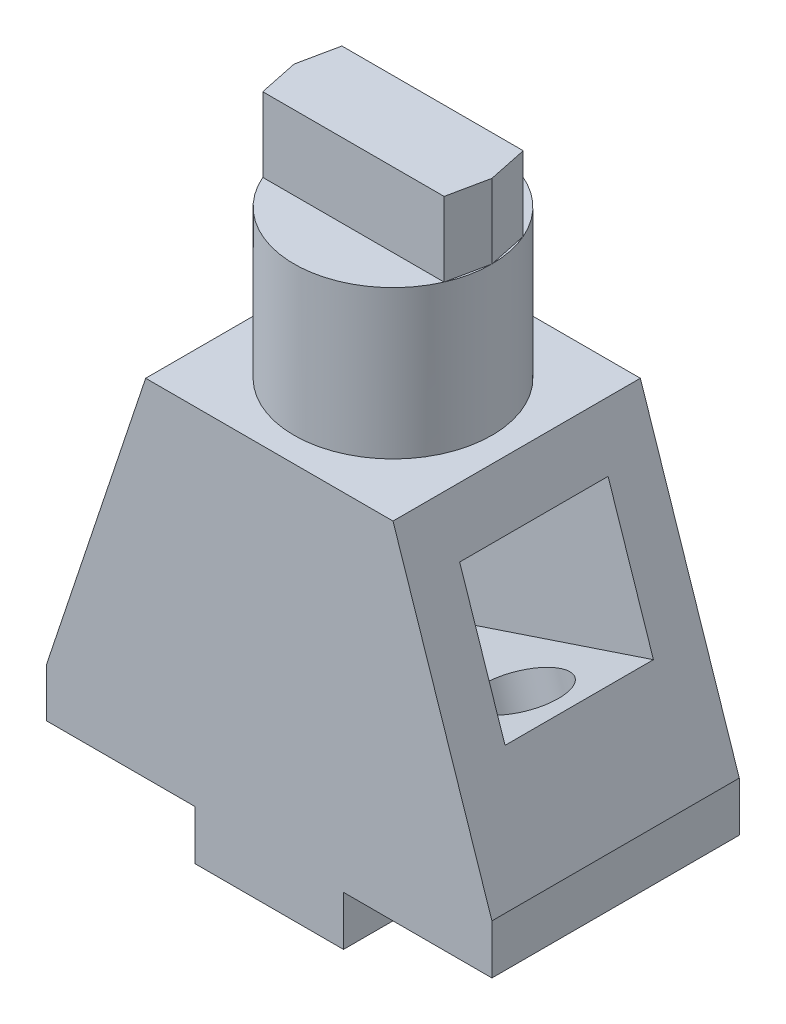
ISO-10303-21;
HEADER;
FILE_DESCRIPTION(('STEP AP214'),'2;1');
FILE_NAME('part.step','',(''),(''),'','','');
FILE_SCHEMA(('AUTOMOTIVE_DESIGN { 1 0 10303 214 1 1 1 1 }'));
ENDSEC;
DATA;
#1=APPLICATION_CONTEXT('core data for automotive mechanical design processes');
#2=APPLICATION_PROTOCOL_DEFINITION('international standard','automotive_design',2000,#1);
#3=PRODUCT_CONTEXT('',#1,'mechanical');
#4=PRODUCT('Part','Part','',(#3));
#5=PRODUCT_RELATED_PRODUCT_CATEGORY('part','',(#4));
#6=PRODUCT_DEFINITION_FORMATION('','',#4);
#7=PRODUCT_DEFINITION_CONTEXT('part definition',#1,'design');
#8=PRODUCT_DEFINITION('design','',#6,#7);
#9=PRODUCT_DEFINITION_SHAPE('','',#8);
#10=(LENGTH_UNIT() NAMED_UNIT(*) SI_UNIT(.MILLI.,.METRE.));
#11=(NAMED_UNIT(*) PLANE_ANGLE_UNIT() SI_UNIT($,.RADIAN.));
#12=(NAMED_UNIT(*) SI_UNIT($,.STERADIAN.) SOLID_ANGLE_UNIT());
#13=UNCERTAINTY_MEASURE_WITH_UNIT(LENGTH_MEASURE(1.E-05),#10,'distance_accuracy_value','');
#14=(GEOMETRIC_REPRESENTATION_CONTEXT(3) GLOBAL_UNCERTAINTY_ASSIGNED_CONTEXT((#13)) GLOBAL_UNIT_ASSIGNED_CONTEXT((#10,
#11,#12)) REPRESENTATION_CONTEXT('',''));
#15=CARTESIAN_POINT('',(0.,0.,0.));
#16=DIRECTION('',(0.,0.,1.));
#17=DIRECTION('',(1.,0.,0.));
#18=AXIS2_PLACEMENT_3D('',#15,#16,#17);
#19=CARTESIAN_POINT('',(45.,100.,-25.));
#20=DIRECTION('',(0.,1.,0.));
#21=DIRECTION('',(0.,0.,1.));
#22=AXIS2_PLACEMENT_3D('',#19,#20,#21);
#23=PLANE('',#22);
#24=DIRECTION('',(0.20430964368922,0.,0.978906312930703));
#25=VECTOR('',#24,1.);
#26=CARTESIAN_POINT('',(26.6696972201766,100.,-17.));
#27=LINE('',#26,#25);
#28=CARTESIAN_POINT('',(25.,100.,-25.));
#29=VERTEX_POINT('',#28);
#30=CARTESIAN_POINT('',(26.6696972201766,100.,-17.));
#31=VERTEX_POINT('',#30);
#32=EDGE_CURVE('E65',#29,#31,#27,.T.);
#33=ORIENTED_EDGE('',*,*,#32,.F.);
#34=CARTESIAN_POINT('',(45.,100.,-25.));
#35=DIRECTION('',(0.,1.,0.));
#36=DIRECTION('',(0.,0.,1.));
#37=AXIS2_PLACEMENT_3D('',#34,#35,#36);
#38=CIRCLE('',#37,20.);
#39=EDGE_CURVE('E209',#29,#31,#38,.T.);
#40=ORIENTED_EDGE('',*,*,#39,.T.);
#41=EDGE_LOOP('',(#33,#40));
#42=FACE_BOUND('',#41,.T.);
#43=ADVANCED_FACE('F39',(#42),#23,.T.);
#44=DIRECTION('',(-0.20430964368922,0.,0.978906312930703));
#45=VECTOR('',#44,1.);
#46=CARTESIAN_POINT('',(25.,100.,-25.));
#47=LINE('',#46,#45);
#48=CARTESIAN_POINT('',(26.6696972201766,100.,-33.));
#49=VERTEX_POINT('',#48);
#50=EDGE_CURVE('E202',#49,#29,#47,.T.);
#51=ORIENTED_EDGE('',*,*,#50,.F.);
#52=EDGE_CURVE('E476',#49,#29,#38,.T.);
#53=ORIENTED_EDGE('',*,*,#52,.T.);
#54=EDGE_LOOP('',(#51,#53));
#55=FACE_BOUND('',#54,.T.);
#56=ADVANCED_FACE('F410',(#55),#23,.T.);
#57=DIRECTION('',(-1.,0.,0.));
#58=VECTOR('',#57,1.);
#59=CARTESIAN_POINT('',(26.6696972201766,100.,-33.));
#60=LINE('',#59,#58);
#61=CARTESIAN_POINT('',(63.3303027798234,100.,-33.));
#62=VERTEX_POINT('',#61);
#63=EDGE_CURVE('E457',#62,#49,#60,.T.);
#64=ORIENTED_EDGE('',*,*,#63,.F.);
#65=EDGE_CURVE('E483',#62,#49,#38,.T.);
#66=ORIENTED_EDGE('',*,*,#65,.T.);
#67=EDGE_LOOP('',(#64,#66));
#68=FACE_BOUND('',#67,.T.);
#69=ADVANCED_FACE('F411',(#68),#23,.T.);
#70=DIRECTION('',(-0.20430964368922,0.,-0.978906312930703));
#71=VECTOR('',#70,1.);
#72=CARTESIAN_POINT('',(63.3303027798234,100.,-33.));
#73=LINE('',#72,#71);
#74=CARTESIAN_POINT('',(65.,100.,-25.));
#75=VERTEX_POINT('',#74);
#76=EDGE_CURVE('E438',#75,#62,#73,.T.);
#77=ORIENTED_EDGE('',*,*,#76,.F.);
#78=EDGE_CURVE('E217',#75,#62,#38,.T.);
#79=ORIENTED_EDGE('',*,*,#78,.T.);
#80=EDGE_LOOP('',(#77,#79));
#81=FACE_BOUND('',#80,.T.);
#82=ADVANCED_FACE('F426',(#81),#23,.T.);
#83=DIRECTION('',(0.20430964368922,0.,-0.978906312930703));
#84=VECTOR('',#83,1.);
#85=CARTESIAN_POINT('',(65.,100.,-25.));
#86=LINE('',#85,#84);
#87=CARTESIAN_POINT('',(63.3303027798234,100.,-17.));
#88=VERTEX_POINT('',#87);
#89=EDGE_CURVE('E434',#88,#75,#86,.T.);
#90=ORIENTED_EDGE('',*,*,#89,.F.);
#91=EDGE_CURVE('E215',#88,#75,#38,.T.);
#92=ORIENTED_EDGE('',*,*,#91,.T.);
#93=EDGE_LOOP('',(#90,#92));
#94=FACE_BOUND('',#93,.T.);
#95=ADVANCED_FACE('F420',(#94),#23,.T.);
#96=CARTESIAN_POINT('',(0.,10.,-50.));
#97=DIRECTION('',(-1.,0.,0.));
#98=DIRECTION('',(0.,0.,1.));
#99=AXIS2_PLACEMENT_3D('',#96,#97,#98);
#100=PLANE('',#99);
#101=DIRECTION('',(0.,1.,0.));
#102=VECTOR('',#101,1.);
#103=CARTESIAN_POINT('',(0.,10.,-10.));
#104=LINE('',#103,#102);
#105=CARTESIAN_POINT('',(0.,4.50296453108829,-10.));
#106=VERTEX_POINT('',#105);
#107=CARTESIAN_POINT('',(0.,10.,-10.));
#108=VERTEX_POINT('',#107);
#109=EDGE_CURVE('E246',#106,#108,#104,.T.);
#110=ORIENTED_EDGE('',*,*,#109,.F.);
#111=DIRECTION('',(0.,0.,1.));
#112=VECTOR('',#111,1.);
#113=CARTESIAN_POINT('',(0.,4.50296453108829,-50.));
#114=LINE('',#113,#112);
#115=CARTESIAN_POINT('',(0.,4.50296453108829,-40.));
#116=VERTEX_POINT('',#115);
#117=EDGE_CURVE('E249',#116,#106,#114,.T.);
#118=ORIENTED_EDGE('',*,*,#117,.F.);
#119=DIRECTION('',(0.,-1.,0.));
#120=VECTOR('',#119,1.);
#121=CARTESIAN_POINT('',(0.,10.,-40.));
#122=LINE('',#121,#120);
#123=CARTESIAN_POINT('',(0.,10.,-40.));
#124=VERTEX_POINT('',#123);
#125=EDGE_CURVE('E241',#124,#116,#122,.T.);
#126=ORIENTED_EDGE('',*,*,#125,.F.);
#127=DIRECTION('',(0.,0.,1.));
#128=VECTOR('',#127,1.);
#129=CARTESIAN_POINT('',(0.,10.,-50.));
#130=LINE('',#129,#128);
#131=CARTESIAN_POINT('',(0.,10.,-50.));
#132=VERTEX_POINT('',#131);
#133=EDGE_CURVE('E48',#132,#124,#130,.T.);
#134=ORIENTED_EDGE('',*,*,#133,.F.);
#135=DIRECTION('',(0.,-1.,0.));
#136=VECTOR('',#135,1.);
#137=CARTESIAN_POINT('',(0.,10.,-50.));
#138=LINE('',#137,#136);
#139=CARTESIAN_POINT('',(0.,0.,-50.));
#140=VERTEX_POINT('',#139);
#141=EDGE_CURVE('E251',#132,#140,#138,.T.);
#142=ORIENTED_EDGE('',*,*,#141,.T.);
#143=DIRECTION('',(0.,0.,1.));
#144=VECTOR('',#143,1.);
#145=CARTESIAN_POINT('',(0.,0.,-50.));
#146=LINE('',#145,#144);
#147=CARTESIAN_POINT('',(0.,0.,0.));
#148=VERTEX_POINT('',#147);
#149=EDGE_CURVE('E43',#140,#148,#146,.T.);
#150=ORIENTED_EDGE('',*,*,#149,.T.);
#151=DIRECTION('',(0.,-1.,0.));
#152=VECTOR('',#151,1.);
#153=CARTESIAN_POINT('',(0.,10.,0.));
#154=LINE('',#153,#152);
#155=CARTESIAN_POINT('',(0.,10.,0.));
#156=VERTEX_POINT('',#155);
#157=EDGE_CURVE('E252',#156,#148,#154,.T.);
#158=ORIENTED_EDGE('',*,*,#157,.F.);
#159=EDGE_CURVE('E314',#108,#156,#130,.T.);
#160=ORIENTED_EDGE('',*,*,#159,.F.);
#161=EDGE_LOOP('',(#110,#118,#126,#134,#142,#150,#158,#160));
#162=FACE_BOUND('',#161,.T.);
#163=ADVANCED_FACE('F41',(#162),#100,.T.);
#164=CARTESIAN_POINT('',(20.,70.,-50.));
#165=DIRECTION('',(-0.948683298050514,0.316227766016838,0.));
#166=DIRECTION('',(-0.316227766016838,-0.948683298050514,0.));
#167=AXIS2_PLACEMENT_3D('',#164,#165,#166);
#168=PLANE('',#167);
#169=DIRECTION('',(0.316227766016838,0.948683298050514,0.));
#170=VECTOR('',#169,1.);
#171=CARTESIAN_POINT('',(20.,70.,-10.));
#172=LINE('',#171,#170);
#173=CARTESIAN_POINT('',(9.40186821726848,38.2056046518055,-10.));
#174=VERTEX_POINT('',#173);
#175=EDGE_CURVE('E248',#108,#174,#172,.T.);
#176=ORIENTED_EDGE('',*,*,#175,.F.);
#177=ORIENTED_EDGE('',*,*,#159,.T.);
#178=DIRECTION('',(-0.316227766016838,-0.948683298050514,0.));
#179=VECTOR('',#178,1.);
#180=CARTESIAN_POINT('',(20.,70.,0.));
#181=LINE('',#180,#179);
#182=CARTESIAN_POINT('',(20.,70.,0.));
#183=VERTEX_POINT('',#182);
#184=EDGE_CURVE('E260',#183,#156,#181,.T.);
#185=ORIENTED_EDGE('',*,*,#184,.F.);
#186=DIRECTION('',(0.,0.,1.));
#187=VECTOR('',#186,1.);
#188=CARTESIAN_POINT('',(20.,70.,-50.));
#189=LINE('',#188,#187);
#190=CARTESIAN_POINT('',(20.,70.,-50.));
#191=VERTEX_POINT('',#190);
#192=EDGE_CURVE('E312',#191,#183,#189,.T.);
#193=ORIENTED_EDGE('',*,*,#192,.F.);
#194=DIRECTION('',(-0.316227766016838,-0.948683298050514,0.));
#195=VECTOR('',#194,1.);
#196=CARTESIAN_POINT('',(20.,70.,-50.));
#197=LINE('',#196,#195);
#198=EDGE_CURVE('E281',#191,#132,#197,.T.);
#199=ORIENTED_EDGE('',*,*,#198,.T.);
#200=ORIENTED_EDGE('',*,*,#133,.T.);
#201=DIRECTION('',(-0.316227766016838,-0.948683298050514,0.));
#202=VECTOR('',#201,1.);
#203=CARTESIAN_POINT('',(20.,70.,-40.));
#204=LINE('',#203,#202);
#205=CARTESIAN_POINT('',(9.40186821726847,38.2056046518054,-40.));
#206=VERTEX_POINT('',#205);
#207=EDGE_CURVE('E231',#206,#124,#204,.T.);
#208=ORIENTED_EDGE('',*,*,#207,.F.);
#209=DIRECTION('',(0.,0.,-1.));
#210=VECTOR('',#209,1.);
#211=CARTESIAN_POINT('',(9.40186821726848,38.2056046518055,-50.));
#212=LINE('',#211,#210);
#213=EDGE_CURVE('E242',#174,#206,#212,.T.);
#214=ORIENTED_EDGE('',*,*,#213,.F.);
#215=EDGE_LOOP('',(#176,#177,#185,#193,#199,#200,#208,#214));
#216=FACE_BOUND('',#215,.T.);
#217=ADVANCED_FACE('F344',(#216),#168,.T.);
#218=CARTESIAN_POINT('',(70.,70.,-50.));
#219=DIRECTION('',(0.,1.,0.));
#220=DIRECTION('',(0.,0.,1.));
#221=AXIS2_PLACEMENT_3D('',#218,#219,#220);
#222=PLANE('',#221);
#223=CARTESIAN_POINT('',(45.,70.,-25.));
#224=DIRECTION('',(0.,1.,0.));
#225=DIRECTION('',(0.,0.,1.));
#226=AXIS2_PLACEMENT_3D('',#223,#224,#225);
#227=CIRCLE('',#226,20.);
#228=CARTESIAN_POINT('',(45.,70.,-4.99999999999999));
#229=VERTEX_POINT('',#228);
#230=EDGE_CURVE('E11',#229,#229,#227,.T.);
#231=ORIENTED_EDGE('',*,*,#230,.F.);
#232=EDGE_LOOP('',(#231));
#233=FACE_BOUND('',#232,.T.);
#234=DIRECTION('',(-1.,0.,0.));
#235=VECTOR('',#234,1.);
#236=CARTESIAN_POINT('',(70.,70.,0.));
#237=LINE('',#236,#235);
#238=CARTESIAN_POINT('',(70.,70.,0.));
#239=VERTEX_POINT('',#238);
#240=EDGE_CURVE('E307',#239,#183,#237,.T.);
#241=ORIENTED_EDGE('',*,*,#240,.F.);
#242=DIRECTION('',(0.,0.,1.));
#243=VECTOR('',#242,1.);
#244=CARTESIAN_POINT('',(70.,70.,-50.));
#245=LINE('',#244,#243);
#246=CARTESIAN_POINT('',(70.,70.,-50.));
#247=VERTEX_POINT('',#246);
#248=EDGE_CURVE('E320',#247,#239,#245,.T.);
#249=ORIENTED_EDGE('',*,*,#248,.F.);
#250=DIRECTION('',(-1.,0.,0.));
#251=VECTOR('',#250,1.);
#252=CARTESIAN_POINT('',(70.,70.,-50.));
#253=LINE('',#252,#251);
#254=EDGE_CURVE('E279',#247,#191,#253,.T.);
#255=ORIENTED_EDGE('',*,*,#254,.T.);
#256=ORIENTED_EDGE('',*,*,#192,.T.);
#257=EDGE_LOOP('',(#241,#249,#255,#256));
#258=FACE_BOUND('',#257,.T.);
#259=ADVANCED_FACE('F393',(#233,#258),#222,.T.);
#260=CARTESIAN_POINT('',(90.,10.,-50.));
#261=DIRECTION('',(0.948683298050514,0.316227766016838,0.));
#262=DIRECTION('',(-0.316227766016838,0.948683298050514,0.));
#263=AXIS2_PLACEMENT_3D('',#260,#261,#262);
#264=PLANE('',#263);
#265=DIRECTION('',(0.,0.,-1.));
#266=VECTOR('',#265,1.);
#267=CARTESIAN_POINT('',(82.6491106406736,32.0526680779795,-40.));
#268=LINE('',#267,#266);
#269=CARTESIAN_POINT('',(82.6491106406736,32.0526680779795,-10.));
#270=VERTEX_POINT('',#269);
#271=CARTESIAN_POINT('',(82.6491106406736,32.0526680779793,-40.));
#272=VERTEX_POINT('',#271);
#273=EDGE_CURVE('E220',#270,#272,#268,.T.);
#274=ORIENTED_EDGE('',*,*,#273,.F.);
#275=DIRECTION('',(0.316227766016837,-0.948683298050514,0.));
#276=VECTOR('',#275,1.);
#277=CARTESIAN_POINT('',(82.6491106406736,32.0526680779795,-10.));
#278=LINE('',#277,#276);
#279=CARTESIAN_POINT('',(73.4785054261853,59.5644837214444,-10.));
#280=VERTEX_POINT('',#279);
#281=EDGE_CURVE('E230',#280,#270,#278,.T.);
#282=ORIENTED_EDGE('',*,*,#281,.F.);
#283=DIRECTION('',(0.,0.,1.));
#284=VECTOR('',#283,1.);
#285=CARTESIAN_POINT('',(73.4785054261853,59.5644837214444,-10.));
#286=LINE('',#285,#284);
#287=CARTESIAN_POINT('',(73.4785054261853,59.5644837214444,-40.));
#288=VERTEX_POINT('',#287);
#289=EDGE_CURVE('E221',#288,#280,#286,.T.);
#290=ORIENTED_EDGE('',*,*,#289,.F.);
#291=DIRECTION('',(-0.316227766016837,0.948683298050514,0.));
#292=VECTOR('',#291,1.);
#293=CARTESIAN_POINT('',(73.4785054261853,59.5644837214444,-40.));
#294=LINE('',#293,#292);
#295=EDGE_CURVE('E222',#272,#288,#294,.T.);
#296=ORIENTED_EDGE('',*,*,#295,.F.);
#297=EDGE_LOOP('',(#274,#282,#290,#296));
#298=FACE_BOUND('',#297,.T.);
#299=DIRECTION('',(-0.316227766016838,0.948683298050514,0.));
#300=VECTOR('',#299,1.);
#301=CARTESIAN_POINT('',(90.,10.,0.));
#302=LINE('',#301,#300);
#303=CARTESIAN_POINT('',(90.,10.,0.));
#304=VERTEX_POINT('',#303);
#305=EDGE_CURVE('E302',#304,#239,#302,.T.);
#306=ORIENTED_EDGE('',*,*,#305,.F.);
#307=DIRECTION('',(0.,0.,1.));
#308=VECTOR('',#307,1.);
#309=CARTESIAN_POINT('',(90.,10.,-50.));
#310=LINE('',#309,#308);
#311=CARTESIAN_POINT('',(90.,10.,-50.));
#312=VERTEX_POINT('',#311);
#313=EDGE_CURVE('E317',#312,#304,#310,.T.);
#314=ORIENTED_EDGE('',*,*,#313,.F.);
#315=DIRECTION('',(-0.316227766016838,0.948683298050514,0.));
#316=VECTOR('',#315,1.);
#317=CARTESIAN_POINT('',(90.,10.,-50.));
#318=LINE('',#317,#316);
#319=EDGE_CURVE('E274',#312,#247,#318,.T.);
#320=ORIENTED_EDGE('',*,*,#319,.T.);
#321=ORIENTED_EDGE('',*,*,#248,.T.);
#322=EDGE_LOOP('',(#306,#314,#320,#321));
#323=FACE_BOUND('',#322,.T.);
#324=ADVANCED_FACE('F361',(#298,#323),#264,.T.);
#325=CARTESIAN_POINT('',(90.,0.,-50.));
#326=DIRECTION('',(1.,0.,0.));
#327=DIRECTION('',(0.,0.,-1.));
#328=AXIS2_PLACEMENT_3D('',#325,#326,#327);
#329=PLANE('',#328);
#330=DIRECTION('',(0.,1.,0.));
#331=VECTOR('',#330,1.);
#332=CARTESIAN_POINT('',(90.,0.,0.));
#333=LINE('',#332,#331);
#334=CARTESIAN_POINT('',(90.,0.,0.));
#335=VERTEX_POINT('',#334);
#336=EDGE_CURVE('E303',#335,#304,#333,.T.);
#337=ORIENTED_EDGE('',*,*,#336,.F.);
#338=DIRECTION('',(0.,0.,1.));
#339=VECTOR('',#338,1.);
#340=CARTESIAN_POINT('',(90.,0.,-50.));
#341=LINE('',#340,#339);
#342=CARTESIAN_POINT('',(90.,0.,-50.));
#343=VERTEX_POINT('',#342);
#344=EDGE_CURVE('E321',#343,#335,#341,.T.);
#345=ORIENTED_EDGE('',*,*,#344,.F.);
#346=DIRECTION('',(0.,1.,0.));
#347=VECTOR('',#346,1.);
#348=CARTESIAN_POINT('',(90.,0.,-50.));
#349=LINE('',#348,#347);
#350=EDGE_CURVE('E275',#343,#312,#349,.T.);
#351=ORIENTED_EDGE('',*,*,#350,.T.);
#352=ORIENTED_EDGE('',*,*,#313,.T.);
#353=EDGE_LOOP('',(#337,#345,#351,#352));
#354=FACE_BOUND('',#353,.T.);
#355=ADVANCED_FACE('F391',(#354),#329,.T.);
#356=CARTESIAN_POINT('',(60.,0.,-50.));
#357=DIRECTION('',(0.,-1.,0.));
#358=DIRECTION('',(0.,0.,-1.));
#359=AXIS2_PLACEMENT_3D('',#356,#357,#358);
#360=PLANE('',#359);
#361=CARTESIAN_POINT('',(80.2265727019644,0.,-25.));
#362=DIRECTION('',(0.,-1.,0.));
#363=DIRECTION('',(-1.,0.,0.));
#364=AXIS2_PLACEMENT_3D('',#361,#362,#363);
#365=ELLIPSE('',#364,8.43274042711569,8.00000000000002);
#366=CARTESIAN_POINT('',(71.7938322748487,0.,-25.));
#367=VERTEX_POINT('',#366);
#368=EDGE_CURVE('E455',#367,#367,#365,.T.);
#369=ORIENTED_EDGE('',*,*,#368,.F.);
#370=EDGE_LOOP('',(#369));
#371=FACE_BOUND('',#370,.T.);
#372=DIRECTION('',(1.,0.,0.));
#373=VECTOR('',#372,1.);
#374=CARTESIAN_POINT('',(60.,0.,0.));
#375=LINE('',#374,#373);
#376=CARTESIAN_POINT('',(60.,0.,0.));
#377=VERTEX_POINT('',#376);
#378=EDGE_CURVE('E297',#377,#335,#375,.T.);
#379=ORIENTED_EDGE('',*,*,#378,.F.);
#380=DIRECTION('',(0.,0.,1.));
#381=VECTOR('',#380,1.);
#382=CARTESIAN_POINT('',(60.,0.,-50.));
#383=LINE('',#382,#381);
#384=CARTESIAN_POINT('',(60.,0.,-50.));
#385=VERTEX_POINT('',#384);
#386=EDGE_CURVE('E323',#385,#377,#383,.T.);
#387=ORIENTED_EDGE('',*,*,#386,.F.);
#388=DIRECTION('',(1.,0.,0.));
#389=VECTOR('',#388,1.);
#390=CARTESIAN_POINT('',(60.,0.,-50.));
#391=LINE('',#390,#389);
#392=EDGE_CURVE('E267',#385,#343,#391,.T.);
#393=ORIENTED_EDGE('',*,*,#392,.T.);
#394=ORIENTED_EDGE('',*,*,#344,.T.);
#395=EDGE_LOOP('',(#379,#387,#393,#394));
#396=FACE_BOUND('',#395,.T.);
#397=ADVANCED_FACE('F390',(#371,#396),#360,.T.);
#398=CARTESIAN_POINT('',(60.,-10.,-50.));
#399=DIRECTION('',(1.,0.,0.));
#400=DIRECTION('',(0.,0.,-1.));
#401=AXIS2_PLACEMENT_3D('',#398,#399,#400);
#402=PLANE('',#401);
#403=DIRECTION('',(0.,1.,0.));
#404=VECTOR('',#403,1.);
#405=CARTESIAN_POINT('',(60.,-10.,0.));
#406=LINE('',#405,#404);
#407=CARTESIAN_POINT('',(60.,-10.,0.));
#408=VERTEX_POINT('',#407);
#409=EDGE_CURVE('E293',#408,#377,#406,.T.);
#410=ORIENTED_EDGE('',*,*,#409,.F.);
#411=DIRECTION('',(0.,0.,1.));
#412=VECTOR('',#411,1.);
#413=CARTESIAN_POINT('',(60.,-10.,-50.));
#414=LINE('',#413,#412);
#415=CARTESIAN_POINT('',(60.,-10.,-50.));
#416=VERTEX_POINT('',#415);
#417=EDGE_CURVE('E324',#416,#408,#414,.T.);
#418=ORIENTED_EDGE('',*,*,#417,.F.);
#419=DIRECTION('',(0.,1.,0.));
#420=VECTOR('',#419,1.);
#421=CARTESIAN_POINT('',(60.,-10.,-50.));
#422=LINE('',#421,#420);
#423=EDGE_CURVE('E266',#416,#385,#422,.T.);
#424=ORIENTED_EDGE('',*,*,#423,.T.);
#425=ORIENTED_EDGE('',*,*,#386,.T.);
#426=EDGE_LOOP('',(#410,#418,#424,#425));
#427=FACE_BOUND('',#426,.T.);
#428=ADVANCED_FACE('F382',(#427),#402,.T.);
#429=CARTESIAN_POINT('',(30.,-10.,-50.));
#430=DIRECTION('',(0.,-1.,0.));
#431=DIRECTION('',(1.,0.,0.));
#432=AXIS2_PLACEMENT_3D('',#429,#430,#431);
#433=PLANE('',#432);
#434=DIRECTION('',(1.,0.,0.));
#435=VECTOR('',#434,1.);
#436=CARTESIAN_POINT('',(30.,-10.,0.));
#437=LINE('',#436,#435);
#438=CARTESIAN_POINT('',(30.,-10.,0.));
#439=VERTEX_POINT('',#438);
#440=EDGE_CURVE('E295',#439,#408,#437,.T.);
#441=ORIENTED_EDGE('',*,*,#440,.F.);
#442=DIRECTION('',(0.,0.,1.));
#443=VECTOR('',#442,1.);
#444=CARTESIAN_POINT('',(30.,-10.,-50.));
#445=LINE('',#444,#443);
#446=CARTESIAN_POINT('',(30.,-10.,-50.));
#447=VERTEX_POINT('',#446);
#448=EDGE_CURVE('E330',#447,#439,#445,.T.);
#449=ORIENTED_EDGE('',*,*,#448,.F.);
#450=DIRECTION('',(1.,0.,0.));
#451=VECTOR('',#450,1.);
#452=CARTESIAN_POINT('',(30.,-10.,-50.));
#453=LINE('',#452,#451);
#454=EDGE_CURVE('E263',#447,#416,#453,.T.);
#455=ORIENTED_EDGE('',*,*,#454,.T.);
#456=ORIENTED_EDGE('',*,*,#417,.T.);
#457=EDGE_LOOP('',(#441,#449,#455,#456));
#458=FACE_BOUND('',#457,.T.);
#459=ADVANCED_FACE('F381',(#458),#433,.T.);
#460=CARTESIAN_POINT('',(30.,0.,-50.));
#461=DIRECTION('',(-1.,0.,0.));
#462=DIRECTION('',(0.,-1.,0.));
#463=AXIS2_PLACEMENT_3D('',#460,#461,#462);
#464=PLANE('',#463);
#465=DIRECTION('',(0.,-1.,0.));
#466=VECTOR('',#465,1.);
#467=CARTESIAN_POINT('',(30.,0.,0.));
#468=LINE('',#467,#466);
#469=CARTESIAN_POINT('',(30.,0.,0.));
#470=VERTEX_POINT('',#469);
#471=EDGE_CURVE('E287',#470,#439,#468,.T.);
#472=ORIENTED_EDGE('',*,*,#471,.F.);
#473=DIRECTION('',(0.,0.,1.));
#474=VECTOR('',#473,1.);
#475=CARTESIAN_POINT('',(30.,0.,-50.));
#476=LINE('',#475,#474);
#477=CARTESIAN_POINT('',(30.,0.,-50.));
#478=VERTEX_POINT('',#477);
#479=EDGE_CURVE('E327',#478,#470,#476,.T.);
#480=ORIENTED_EDGE('',*,*,#479,.F.);
#481=DIRECTION('',(0.,-1.,0.));
#482=VECTOR('',#481,1.);
#483=CARTESIAN_POINT('',(30.,0.,-50.));
#484=LINE('',#483,#482);
#485=EDGE_CURVE('E257',#478,#447,#484,.T.);
#486=ORIENTED_EDGE('',*,*,#485,.T.);
#487=ORIENTED_EDGE('',*,*,#448,.T.);
#488=EDGE_LOOP('',(#472,#480,#486,#487));
#489=FACE_BOUND('',#488,.T.);
#490=ADVANCED_FACE('F380',(#489),#464,.T.);
#491=CARTESIAN_POINT('',(0.,0.,-50.));
#492=DIRECTION('',(0.,-1.,0.));
#493=DIRECTION('',(0.,0.,-1.));
#494=AXIS2_PLACEMENT_3D('',#491,#492,#493);
#495=PLANE('',#494);
#496=DIRECTION('',(1.,0.,0.));
#497=VECTOR('',#496,1.);
#498=CARTESIAN_POINT('',(0.,0.,0.));
#499=LINE('',#498,#497);
#500=EDGE_CURVE('E288',#148,#470,#499,.T.);
#501=ORIENTED_EDGE('',*,*,#500,.F.);
#502=ORIENTED_EDGE('',*,*,#149,.F.);
#503=DIRECTION('',(1.,0.,0.));
#504=VECTOR('',#503,1.);
#505=CARTESIAN_POINT('',(0.,0.,-50.));
#506=LINE('',#505,#504);
#507=EDGE_CURVE('E258',#140,#478,#506,.T.);
#508=ORIENTED_EDGE('',*,*,#507,.T.);
#509=ORIENTED_EDGE('',*,*,#479,.T.);
#510=EDGE_LOOP('',(#501,#502,#508,#509));
#511=FACE_BOUND('',#510,.T.);
#512=ADVANCED_FACE('F337',(#511),#495,.T.);
#513=CARTESIAN_POINT('',(0.,0.,-50.));
#514=DIRECTION('',(0.,0.,1.));
#515=DIRECTION('',(1.,0.,0.));
#516=AXIS2_PLACEMENT_3D('',#513,#514,#515);
#517=PLANE('',#516);
#518=ORIENTED_EDGE('',*,*,#141,.F.);
#519=ORIENTED_EDGE('',*,*,#198,.F.);
#520=ORIENTED_EDGE('',*,*,#254,.F.);
#521=ORIENTED_EDGE('',*,*,#319,.F.);
#522=ORIENTED_EDGE('',*,*,#350,.F.);
#523=ORIENTED_EDGE('',*,*,#392,.F.);
#524=ORIENTED_EDGE('',*,*,#423,.F.);
#525=ORIENTED_EDGE('',*,*,#454,.F.);
#526=ORIENTED_EDGE('',*,*,#485,.F.);
#527=ORIENTED_EDGE('',*,*,#507,.F.);
#528=EDGE_LOOP('',(#518,#519,#520,#521,#522,#523,#524,#525,#526,#527));
#529=FACE_BOUND('',#528,.T.);
#530=ADVANCED_FACE('F371',(#529),#517,.F.);
#531=CARTESIAN_POINT('',(0.,0.,0.));
#532=DIRECTION('',(0.,0.,1.));
#533=DIRECTION('',(1.,0.,0.));
#534=AXIS2_PLACEMENT_3D('',#531,#532,#533);
#535=PLANE('',#534);
#536=ORIENTED_EDGE('',*,*,#157,.T.);
#537=ORIENTED_EDGE('',*,*,#500,.T.);
#538=ORIENTED_EDGE('',*,*,#471,.T.);
#539=ORIENTED_EDGE('',*,*,#440,.T.);
#540=ORIENTED_EDGE('',*,*,#409,.T.);
#541=ORIENTED_EDGE('',*,*,#378,.T.);
#542=ORIENTED_EDGE('',*,*,#336,.T.);
#543=ORIENTED_EDGE('',*,*,#305,.T.);
#544=ORIENTED_EDGE('',*,*,#240,.T.);
#545=ORIENTED_EDGE('',*,*,#184,.T.);
#546=EDGE_LOOP('',(#536,#537,#538,#539,#540,#541,#542,#543,#544,#545));
#547=FACE_BOUND('',#546,.T.);
#548=ADVANCED_FACE('F339',(#547),#535,.T.);
#549=CARTESIAN_POINT('',(-4.35088935932652,3.05266807797945,-40.));
#550=DIRECTION('',(0.316227766016838,-0.948683298050514,0.));
#551=DIRECTION('',(0.948683298050514,0.316227766016838,0.));
#552=AXIS2_PLACEMENT_3D('',#549,#550,#551);
#553=PLANE('',#552);
#554=CARTESIAN_POINT('',(70.8530260724415,28.1206398885688,-25.));
#555=DIRECTION('',(-0.316227766016838,0.948683298050514,0.));
#556=DIRECTION('',(-0.948683298050514,-0.316227766016838,0.));
#557=AXIS2_PLACEMENT_3D('',#554,#555,#556);
#558=CIRCLE('',#557,8.00000000000002);
#559=CARTESIAN_POINT('',(63.2635596880374,25.5908177604341,-25.));
#560=VERTEX_POINT('',#559);
#561=EDGE_CURVE('E710',#560,#560,#558,.T.);
#562=ORIENTED_EDGE('',*,*,#561,.F.);
#563=EDGE_LOOP('',(#562));
#564=FACE_BOUND('',#563,.T.);
#565=ORIENTED_EDGE('',*,*,#117,.T.);
#566=DIRECTION('',(0.948683298050514,0.316227766016838,0.));
#567=VECTOR('',#566,1.);
#568=CARTESIAN_POINT('',(-4.35088935932652,3.05266807797945,-10.));
#569=LINE('',#568,#567);
#570=EDGE_CURVE('E233',#106,#270,#569,.T.);
#571=ORIENTED_EDGE('',*,*,#570,.T.);
#572=ORIENTED_EDGE('',*,*,#273,.T.);
#573=DIRECTION('',(0.948683298050514,0.316227766016838,0.));
#574=VECTOR('',#573,1.);
#575=CARTESIAN_POINT('',(-4.35088935932652,3.05266807797945,-40.));
#576=LINE('',#575,#574);
#577=EDGE_CURVE('E229',#116,#272,#576,.T.);
#578=ORIENTED_EDGE('',*,*,#577,.F.);
#579=EDGE_LOOP('',(#565,#571,#572,#578));
#580=FACE_BOUND('',#579,.T.);
#581=ADVANCED_FACE('F358',(#564,#580),#553,.F.);
#582=CARTESIAN_POINT('',(-4.35088935932652,3.05266807797945,-10.));
#583=DIRECTION('',(0.,0.,1.));
#584=DIRECTION('',(1.,0.,0.));
#585=AXIS2_PLACEMENT_3D('',#582,#583,#584);
#586=PLANE('',#585);
#587=ORIENTED_EDGE('',*,*,#109,.T.);
#588=ORIENTED_EDGE('',*,*,#175,.T.);
#589=DIRECTION('',(0.948683298050514,0.316227766016838,0.));
#590=VECTOR('',#589,1.);
#591=CARTESIAN_POINT('',(-13.5214945738148,30.5644837214444,-10.));
#592=LINE('',#591,#590);
#593=EDGE_CURVE('E232',#174,#280,#592,.T.);
#594=ORIENTED_EDGE('',*,*,#593,.T.);
#595=ORIENTED_EDGE('',*,*,#281,.T.);
#596=ORIENTED_EDGE('',*,*,#570,.F.);
#597=EDGE_LOOP('',(#587,#588,#594,#595,#596));
#598=FACE_BOUND('',#597,.T.);
#599=ADVANCED_FACE('F351',(#598),#586,.F.);
#600=CARTESIAN_POINT('',(-13.5214945738148,30.5644837214444,-10.));
#601=DIRECTION('',(-0.316227766016838,0.948683298050514,0.));
#602=DIRECTION('',(-0.948683298050514,-0.316227766016838,0.));
#603=AXIS2_PLACEMENT_3D('',#600,#601,#602);
#604=PLANE('',#603);
#605=ORIENTED_EDGE('',*,*,#213,.T.);
#606=DIRECTION('',(0.948683298050514,0.316227766016838,0.));
#607=VECTOR('',#606,1.);
#608=CARTESIAN_POINT('',(-13.5214945738148,30.5644837214444,-40.));
#609=LINE('',#608,#607);
#610=EDGE_CURVE('E237',#206,#288,#609,.T.);
#611=ORIENTED_EDGE('',*,*,#610,.T.);
#612=ORIENTED_EDGE('',*,*,#289,.T.);
#613=ORIENTED_EDGE('',*,*,#593,.F.);
#614=EDGE_LOOP('',(#605,#611,#612,#613));
#615=FACE_BOUND('',#614,.T.);
#616=ADVANCED_FACE('F368',(#615),#604,.F.);
#617=CARTESIAN_POINT('',(-13.5214945738148,30.5644837214444,-40.));
#618=DIRECTION('',(0.,0.,-1.));
#619=DIRECTION('',(0.,1.,0.));
#620=AXIS2_PLACEMENT_3D('',#617,#618,#619);
#621=PLANE('',#620);
#622=ORIENTED_EDGE('',*,*,#125,.T.);
#623=ORIENTED_EDGE('',*,*,#577,.T.);
#624=ORIENTED_EDGE('',*,*,#295,.T.);
#625=ORIENTED_EDGE('',*,*,#610,.F.);
#626=ORIENTED_EDGE('',*,*,#207,.T.);
#627=EDGE_LOOP('',(#622,#623,#624,#625,#626));
#628=FACE_BOUND('',#627,.T.);
#629=ADVANCED_FACE('F359',(#628),#621,.F.);
#630=CARTESIAN_POINT('',(45.,100.,-25.));
#631=DIRECTION('',(0.,-1.,0.));
#632=DIRECTION('',(0.,0.,-1.));
#633=AXIS2_PLACEMENT_3D('',#630,#631,#632);
#634=CYLINDRICAL_SURFACE('',#633,20.);
#635=ORIENTED_EDGE('',*,*,#91,.F.);
#636=EDGE_CURVE('E208',#31,#88,#38,.T.);
#637=ORIENTED_EDGE('',*,*,#636,.F.);
#638=ORIENTED_EDGE('',*,*,#39,.F.);
#639=ORIENTED_EDGE('',*,*,#52,.F.);
#640=ORIENTED_EDGE('',*,*,#65,.F.);
#641=ORIENTED_EDGE('',*,*,#78,.F.);
#642=EDGE_LOOP('',(#635,#637,#638,#639,#640,#641));
#643=FACE_BOUND('',#642,.T.);
#644=ORIENTED_EDGE('',*,*,#230,.T.);
#645=EDGE_LOOP('',(#644));
#646=FACE_BOUND('',#645,.T.);
#647=ADVANCED_FACE('F416',(#643,#646),#634,.T.);
#648=DIRECTION('',(1.,0.,0.));
#649=VECTOR('',#648,1.);
#650=CARTESIAN_POINT('',(63.3303027798234,100.,-17.));
#651=LINE('',#650,#649);
#652=EDGE_CURVE('E54',#31,#88,#651,.T.);
#653=ORIENTED_EDGE('',*,*,#652,.F.);
#654=ORIENTED_EDGE('',*,*,#636,.T.);
#655=EDGE_LOOP('',(#653,#654));
#656=FACE_BOUND('',#655,.T.);
#657=ADVANCED_FACE('F408',(#656),#23,.T.);
#658=CARTESIAN_POINT('',(26.6696972201766,115.,-17.));
#659=DIRECTION('',(0.978906312930703,0.,-0.20430964368922));
#660=DIRECTION('',(-0.20430964368922,0.,-0.978906312930703));
#661=AXIS2_PLACEMENT_3D('',#658,#659,#660);
#662=PLANE('',#661);
#663=ORIENTED_EDGE('',*,*,#32,.T.);
#664=DIRECTION('',(0.,-1.,0.));
#665=VECTOR('',#664,1.);
#666=CARTESIAN_POINT('',(26.6696972201766,115.,-17.));
#667=LINE('',#666,#665);
#668=CARTESIAN_POINT('',(26.6696972201766,115.,-17.));
#669=VERTEX_POINT('',#668);
#670=EDGE_CURVE('E189',#669,#31,#667,.T.);
#671=ORIENTED_EDGE('',*,*,#670,.F.);
#672=DIRECTION('',(0.20430964368922,0.,0.978906312930703));
#673=VECTOR('',#672,1.);
#674=CARTESIAN_POINT('',(26.6696972201766,115.,-17.));
#675=LINE('',#674,#673);
#676=CARTESIAN_POINT('',(25.,115.,-25.));
#677=VERTEX_POINT('',#676);
#678=EDGE_CURVE('E198',#677,#669,#675,.T.);
#679=ORIENTED_EDGE('',*,*,#678,.F.);
#680=DIRECTION('',(0.,-1.,0.));
#681=VECTOR('',#680,1.);
#682=CARTESIAN_POINT('',(25.,115.,-25.));
#683=LINE('',#682,#681);
#684=EDGE_CURVE('E453',#677,#29,#683,.T.);
#685=ORIENTED_EDGE('',*,*,#684,.T.);
#686=EDGE_LOOP('',(#663,#671,#679,#685));
#687=FACE_BOUND('',#686,.T.);
#688=ADVANCED_FACE('F210',(#687),#662,.F.);
#689=CARTESIAN_POINT('',(63.3303027798234,115.,-17.));
#690=DIRECTION('',(0.,0.,-1.));
#691=DIRECTION('',(-1.,0.,0.));
#692=AXIS2_PLACEMENT_3D('',#689,#690,#691);
#693=PLANE('',#692);
#694=ORIENTED_EDGE('',*,*,#652,.T.);
#695=DIRECTION('',(0.,-1.,0.));
#696=VECTOR('',#695,1.);
#697=CARTESIAN_POINT('',(63.3303027798234,115.,-17.));
#698=LINE('',#697,#696);
#699=CARTESIAN_POINT('',(63.3303027798234,115.,-17.));
#700=VERTEX_POINT('',#699);
#701=EDGE_CURVE('E195',#700,#88,#698,.T.);
#702=ORIENTED_EDGE('',*,*,#701,.F.);
#703=DIRECTION('',(1.,0.,0.));
#704=VECTOR('',#703,1.);
#705=CARTESIAN_POINT('',(63.3303027798234,115.,-17.));
#706=LINE('',#705,#704);
#707=EDGE_CURVE('E186',#669,#700,#706,.T.);
#708=ORIENTED_EDGE('',*,*,#707,.F.);
#709=ORIENTED_EDGE('',*,*,#670,.T.);
#710=EDGE_LOOP('',(#694,#702,#708,#709));
#711=FACE_BOUND('',#710,.T.);
#712=ADVANCED_FACE('F187',(#711),#693,.F.);
#713=CARTESIAN_POINT('',(65.,115.,-25.));
#714=DIRECTION('',(-0.978906312930703,0.,-0.20430964368922));
#715=DIRECTION('',(-0.20430964368922,0.,0.978906312930703));
#716=AXIS2_PLACEMENT_3D('',#713,#714,#715);
#717=PLANE('',#716);
#718=ORIENTED_EDGE('',*,*,#89,.T.);
#719=DIRECTION('',(0.,-1.,0.));
#720=VECTOR('',#719,1.);
#721=CARTESIAN_POINT('',(65.,115.,-25.));
#722=LINE('',#721,#720);
#723=CARTESIAN_POINT('',(65.,115.,-25.));
#724=VERTEX_POINT('',#723);
#725=EDGE_CURVE('E213',#724,#75,#722,.T.);
#726=ORIENTED_EDGE('',*,*,#725,.F.);
#727=DIRECTION('',(0.20430964368922,0.,-0.978906312930703));
#728=VECTOR('',#727,1.);
#729=CARTESIAN_POINT('',(65.,115.,-25.));
#730=LINE('',#729,#728);
#731=EDGE_CURVE('E194',#700,#724,#730,.T.);
#732=ORIENTED_EDGE('',*,*,#731,.F.);
#733=ORIENTED_EDGE('',*,*,#701,.T.);
#734=EDGE_LOOP('',(#718,#726,#732,#733));
#735=FACE_BOUND('',#734,.T.);
#736=ADVANCED_FACE('F445',(#735),#717,.F.);
#737=CARTESIAN_POINT('',(63.3303027798234,115.,-33.));
#738=DIRECTION('',(-0.978906312930703,0.,0.20430964368922));
#739=DIRECTION('',(0.20430964368922,0.,0.978906312930703));
#740=AXIS2_PLACEMENT_3D('',#737,#738,#739);
#741=PLANE('',#740);
#742=ORIENTED_EDGE('',*,*,#76,.T.);
#743=DIRECTION('',(0.,-1.,0.));
#744=VECTOR('',#743,1.);
#745=CARTESIAN_POINT('',(63.3303027798234,115.,-33.));
#746=LINE('',#745,#744);
#747=CARTESIAN_POINT('',(63.3303027798234,115.,-33.));
#748=VERTEX_POINT('',#747);
#749=EDGE_CURVE('E464',#748,#62,#746,.T.);
#750=ORIENTED_EDGE('',*,*,#749,.F.);
#751=DIRECTION('',(-0.20430964368922,0.,-0.978906312930703));
#752=VECTOR('',#751,1.);
#753=CARTESIAN_POINT('',(63.3303027798234,115.,-33.));
#754=LINE('',#753,#752);
#755=EDGE_CURVE('E441',#724,#748,#754,.T.);
#756=ORIENTED_EDGE('',*,*,#755,.F.);
#757=ORIENTED_EDGE('',*,*,#725,.T.);
#758=EDGE_LOOP('',(#742,#750,#756,#757));
#759=FACE_BOUND('',#758,.T.);
#760=ADVANCED_FACE('F466',(#759),#741,.F.);
#761=CARTESIAN_POINT('',(26.6696972201766,115.,-33.));
#762=DIRECTION('',(0.,0.,1.));
#763=DIRECTION('',(1.,0.,0.));
#764=AXIS2_PLACEMENT_3D('',#761,#762,#763);
#765=PLANE('',#764);
#766=ORIENTED_EDGE('',*,*,#63,.T.);
#767=DIRECTION('',(0.,-1.,0.));
#768=VECTOR('',#767,1.);
#769=CARTESIAN_POINT('',(26.6696972201766,115.,-33.));
#770=LINE('',#769,#768);
#771=CARTESIAN_POINT('',(26.6696972201766,115.,-33.));
#772=VERTEX_POINT('',#771);
#773=EDGE_CURVE('E465',#772,#49,#770,.T.);
#774=ORIENTED_EDGE('',*,*,#773,.F.);
#775=DIRECTION('',(-1.,0.,0.));
#776=VECTOR('',#775,1.);
#777=CARTESIAN_POINT('',(26.6696972201766,115.,-33.));
#778=LINE('',#777,#776);
#779=EDGE_CURVE('E446',#748,#772,#778,.T.);
#780=ORIENTED_EDGE('',*,*,#779,.F.);
#781=ORIENTED_EDGE('',*,*,#749,.T.);
#782=EDGE_LOOP('',(#766,#774,#780,#781));
#783=FACE_BOUND('',#782,.T.);
#784=ADVANCED_FACE('F471',(#783),#765,.F.);
#785=CARTESIAN_POINT('',(25.,115.,-25.));
#786=DIRECTION('',(0.978906312930703,0.,0.20430964368922));
#787=DIRECTION('',(0.20430964368922,0.,-0.978906312930703));
#788=AXIS2_PLACEMENT_3D('',#785,#786,#787);
#789=PLANE('',#788);
#790=ORIENTED_EDGE('',*,*,#50,.T.);
#791=ORIENTED_EDGE('',*,*,#684,.F.);
#792=DIRECTION('',(-0.20430964368922,0.,0.978906312930703));
#793=VECTOR('',#792,1.);
#794=CARTESIAN_POINT('',(25.,115.,-25.));
#795=LINE('',#794,#793);
#796=EDGE_CURVE('E203',#772,#677,#795,.T.);
#797=ORIENTED_EDGE('',*,*,#796,.F.);
#798=ORIENTED_EDGE('',*,*,#773,.T.);
#799=EDGE_LOOP('',(#790,#791,#797,#798));
#800=FACE_BOUND('',#799,.T.);
#801=ADVANCED_FACE('F474',(#800),#789,.F.);
#802=CARTESIAN_POINT('',(0.,115.,0.));
#803=DIRECTION('',(0.,-1.,0.));
#804=DIRECTION('',(0.,0.,-1.));
#805=AXIS2_PLACEMENT_3D('',#802,#803,#804);
#806=PLANE('',#805);
#807=ORIENTED_EDGE('',*,*,#678,.T.);
#808=ORIENTED_EDGE('',*,*,#707,.T.);
#809=ORIENTED_EDGE('',*,*,#731,.T.);
#810=ORIENTED_EDGE('',*,*,#755,.T.);
#811=ORIENTED_EDGE('',*,*,#779,.T.);
#812=ORIENTED_EDGE('',*,*,#796,.T.);
#813=EDGE_LOOP('',(#807,#808,#809,#810,#811,#812));
#814=FACE_BOUND('',#813,.T.);
#815=ADVANCED_FACE('F200',(#814),#806,.F.);
#816=CARTESIAN_POINT('',(84.203915431768,-11.9320281894107,-25.));
#817=DIRECTION('',(-0.316227766016838,0.948683298050514,0.));
#818=DIRECTION('',(-0.948683298050514,-0.316227766016838,0.));
#819=AXIS2_PLACEMENT_3D('',#816,#817,#818);
#820=CYLINDRICAL_SURFACE('',#819,8.00000000000002);
#821=ORIENTED_EDGE('',*,*,#368,.T.);
#822=EDGE_LOOP('',(#821));
#823=FACE_BOUND('',#822,.T.);
#824=ORIENTED_EDGE('',*,*,#561,.T.);
#825=EDGE_LOOP('',(#824));
#826=FACE_BOUND('',#825,.T.);
#827=ADVANCED_FACE('F562',(#823,#826),#820,.F.);
#828=CLOSED_SHELL('',(#43,#56,#69,#82,#95,#163,#217,#259,#324,#355,#397,#428,#459,#490,#512,
#530,#548,#581,#599,#616,#629,#647,#657,#688,#712,#736,#760,#784,#801,#815,#827));
#829=MANIFOLD_SOLID_BREP('B2',#828);
#830=ADVANCED_BREP_SHAPE_REPRESENTATION('',(#18,#829),#14);
#831=SHAPE_DEFINITION_REPRESENTATION(#9,#830);
ENDSEC;
END-ISO-10303-21;
